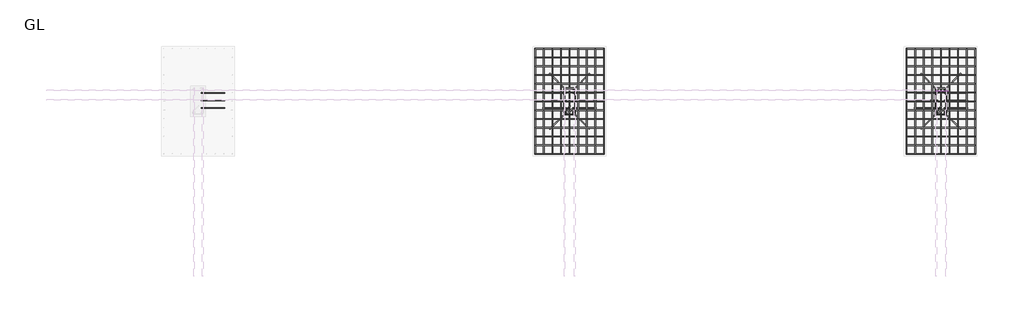
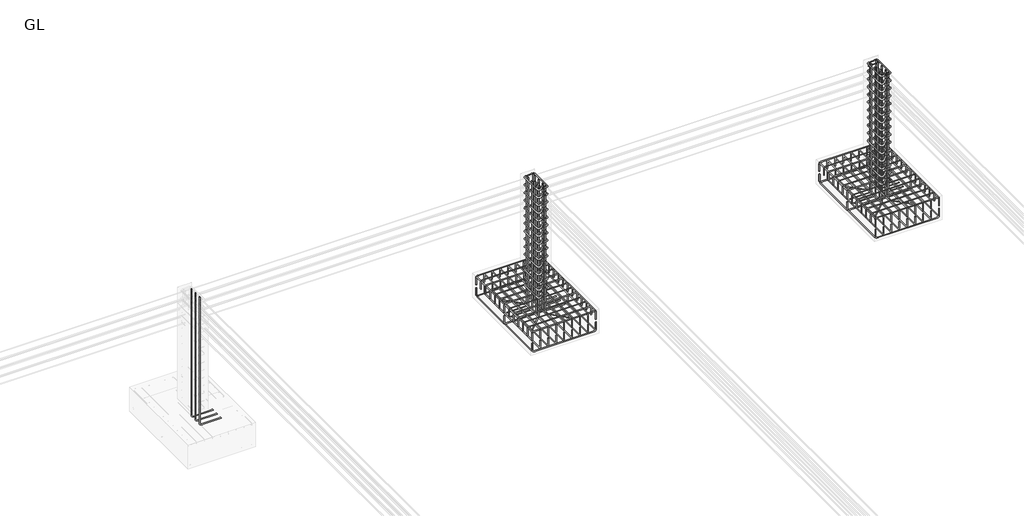
# One storey, part 16 of 16: 24 reinforcing bars.
"""IFC4 building model written with IfcOpenShell, lengths in millimetres."""

from ifc_helpers import new_model, si_unit, point, frame, origin, place, context, project, spatial, polyline, circle_curve, trimmed, segment, composite_curve, source, transform, mapped, element, save
from ifc_brep_helpers import swept_disk

model = new_model("IFC4")

# Units and contexts
model_context = context("Model", 3, world=origin())
ifc_project = project(units=[si_unit("LENGTHUNIT", "METRE", prefix="MILLI")], contexts=[model_context])

# Site, building, storey
site = spatial("IfcSite", under=ifc_project)
building = spatial("IfcBuilding", under=site)
storey = spatial("IfcBuildingStorey", under=building, Name="GL", Elevation=-1829.0)

# Reinforcing bars
placement = place(None, origin())
reinforcing_bar_shape = source(origin(), model_context, "Body", "SolidModel", [
    swept_disk(composite_curve([segment(polyline([(2141.0455621, 4968.8832479, -2089.0), (2141.0455621, 4968.8832479, -2213.0)]), True, "CONTINUOUS"), segment(trimmed(circle_curve(frame((2111.0455621, 4968.8832479, -2213.0), z_axis=(0.0, 1.0, 0.0), x_axis=(30.0, 0.0, 0.0)), 30.0), [point((2141.0455621, 4968.8832479, -2213.0))], [point((2111.0455621, 4968.8832479, -2243.0))], True, "CARTESIAN"), True, "CONTINUOUS"), segment(polyline([(2111.0455621, 4968.8832479, -2243.0), (1043.0455621, 4968.8832479, -2243.0)]), True, "CONTINUOUS"), segment(trimmed(circle_curve(frame((1043.0455621, 4968.8832479, -2213.0), z_axis=(0.0, 1.0, 0.0), x_axis=(0.0, 0.0, -30.0)), 30.0), [point((1043.0455621, 4968.8832479, -2243.0))], [point((1013.0455621, 4968.8832479, -2213.0))], True, "CARTESIAN"), True, "CONTINUOUS"), segment(polyline([(1013.0455621, 4968.8832479, -2213.0), (1013.0455621, 4968.8832479, -2089.0)]), True, "CONTINUOUS")], self_intersect=False), 6.0),
])
element("IfcReinforcingBar", 1, at=placement, inside=storey, context=model_context, shape_type="MappedRepresentation", body=[
    mapped(reinforcing_bar_shape, transform((0.0, 0.0, 0.0), x_axis=(1.0, 0.0, 0.0), y_axis=(0.0, 1.0, 0.0), z_axis=(0.0, 0.0, 1.0))),
    mapped(reinforcing_bar_shape, transform((0.0, -864.0, 0.0), x_axis=(1.0, 0.0, 0.0), y_axis=(0.0, 1.0, 0.0), z_axis=(0.0, 0.0, 1.0))),
    mapped(reinforcing_bar_shape, transform((0.0, -1728.0, 0.0), x_axis=(1.0, 0.0, 0.0), y_axis=(0.0, 1.0, 0.0), z_axis=(0.0, 0.0, 1.0))),
])
reinforcing_bar_2_shape = source(origin(), model_context, "Body", "SolidModel", [
    swept_disk(composite_curve([segment(polyline([(1013.0455621, 4968.8832479, -2022.436678), (1013.0455621, 4968.8832479, -1898.436678)]), True, "CONTINUOUS"), segment(trimmed(circle_curve(frame((1043.0455621, 4968.8832479, -1898.436678), z_axis=(0.0, 1.0, 0.0), x_axis=(-30.000000000000114, 0.0, 0.0)), 30.0), [point((1013.0455621, 4968.8832479, -1898.436678))], [point((1043.0455621, 4968.8832479, -1868.436678))], True, "CARTESIAN"), True, "CONTINUOUS"), segment(polyline([(1043.0455621, 4968.8832479, -1868.436678), (2111.0455621, 4968.8832479, -1868.436678)]), True, "CONTINUOUS"), segment(trimmed(circle_curve(frame((2111.0455621, 4968.8832479, -1898.436678), z_axis=(0.0, 1.0, 0.0), x_axis=(0.0, 0.0, 30.0)), 30.0), [point((2111.0455621, 4968.8832479, -1868.436678))], [point((2141.0455621, 4968.8832479, -1898.436678))], True, "CARTESIAN"), True, "CONTINUOUS"), segment(polyline([(2141.0455621, 4968.8832479, -1898.436678), (2141.0455621, 4968.8832479, -2022.436678)]), True, "CONTINUOUS")], self_intersect=False), 6.0),
])
element("IfcReinforcingBar", 2, at=placement, inside=storey, context=model_context, shape_type="MappedRepresentation", body=[
    mapped(reinforcing_bar_2_shape, transform((0.0, 0.0, 0.0), x_axis=(1.0, 0.0, 0.0), y_axis=(0.0, 1.0, 0.0), z_axis=(0.0, 0.0, 1.0))),
    mapped(reinforcing_bar_2_shape, transform((0.0, -144.0, 0.0), x_axis=(1.0, 0.0, 0.0), y_axis=(0.0, 1.0, 0.0), z_axis=(0.0, 0.0, 1.0))),
    mapped(reinforcing_bar_2_shape, transform((0.0, -288.0, 0.0), x_axis=(1.0, 0.0, 0.0), y_axis=(0.0, 1.0, 0.0), z_axis=(0.0, 0.0, 1.0))),
    mapped(reinforcing_bar_2_shape, transform((0.0, -432.0, 0.0), x_axis=(1.0, 0.0, 0.0), y_axis=(0.0, 1.0, 0.0), z_axis=(0.0, 0.0, 1.0))),
    mapped(reinforcing_bar_2_shape, transform((0.0, -576.0, 0.0), x_axis=(1.0, 0.0, 0.0), y_axis=(0.0, 1.0, 0.0), z_axis=(0.0, 0.0, 1.0))),
    mapped(reinforcing_bar_2_shape, transform((0.0, -720.0, 0.0), x_axis=(1.0, 0.0, 0.0), y_axis=(0.0, 1.0, 0.0), z_axis=(0.0, 0.0, 1.0))),
    mapped(reinforcing_bar_2_shape, transform((0.0, -864.0, 0.0), x_axis=(1.0, 0.0, 0.0), y_axis=(0.0, 1.0, 0.0), z_axis=(0.0, 0.0, 1.0))),
    mapped(reinforcing_bar_2_shape, transform((0.0, -1008.0, 0.0), x_axis=(1.0, 0.0, 0.0), y_axis=(0.0, 1.0, 0.0), z_axis=(0.0, 0.0, 1.0))),
    mapped(reinforcing_bar_2_shape, transform((0.0, -1152.0, 0.0), x_axis=(1.0, 0.0, 0.0), y_axis=(0.0, 1.0, 0.0), z_axis=(0.0, 0.0, 1.0))),
    mapped(reinforcing_bar_2_shape, transform((0.0, -1296.0, 0.0), x_axis=(1.0, 0.0, 0.0), y_axis=(0.0, 1.0, 0.0), z_axis=(0.0, 0.0, 1.0))),
    mapped(reinforcing_bar_2_shape, transform((0.0, -1440.0, 0.0), x_axis=(1.0, 0.0, 0.0), y_axis=(0.0, 1.0, 0.0), z_axis=(0.0, 0.0, 1.0))),
    mapped(reinforcing_bar_2_shape, transform((0.0, -1584.0, 0.0), x_axis=(1.0, 0.0, 0.0), y_axis=(0.0, 1.0, 0.0), z_axis=(0.0, 0.0, 1.0))),
    mapped(reinforcing_bar_2_shape, transform((0.0, -1728.0, 0.0), x_axis=(1.0, 0.0, 0.0), y_axis=(0.0, 1.0, 0.0), z_axis=(0.0, 0.0, 1.0))),
])
reinforcing_bar_3_shape = source(origin(), model_context, "Body", "SolidModel", [
    swept_disk(composite_curve([segment(polyline([(1013.0455621, 3240.8832479, -2027.5081232), (1013.0455621, 3240.8832479, -1903.5081232)]), True, "CONTINUOUS"), segment(trimmed(circle_curve(frame((1013.0455621, 3270.8832479, -1903.5081232), z_axis=(-1.0, 0.0, 0.0), x_axis=(0.0, -30.0, 0.0)), 30.0), [point((1013.0455621, 3240.8832479, -1903.5081232))], [point((1013.0455621, 3270.8832479, -1873.5081232))], True, "CARTESIAN"), True, "CONTINUOUS"), segment(polyline([(1013.0455621, 3270.8832479, -1873.5081232), (1013.0455621, 4938.8832479, -1873.5081232)]), True, "CONTINUOUS"), segment(trimmed(circle_curve(frame((1013.0455621, 4938.8832479, -1903.5081232), z_axis=(-1.0, 0.0, 0.0), x_axis=(0.0, 0.0, 30.0)), 30.0), [point((1013.0455621, 4938.8832479, -1873.5081232))], [point((1013.0455621, 4968.8832479, -1903.5081232))], True, "CARTESIAN"), True, "CONTINUOUS"), segment(polyline([(1013.0455621, 4968.8832479, -1903.5081232), (1013.0455621, 4968.8832479, -2027.5081232)]), True, "CONTINUOUS")], self_intersect=False), 6.0),
])
element("IfcReinforcingBar", 3, at=placement, inside=storey, context=model_context, shape_type="MappedRepresentation", body=[
    mapped(reinforcing_bar_3_shape, transform((0.0, 0.0, 0.0), x_axis=(1.0, 0.0, 0.0), y_axis=(0.0, 1.0, 0.0), z_axis=(0.0, 0.0, 1.0))),
    mapped(reinforcing_bar_3_shape, transform((141.0, 0.0, 0.0), x_axis=(1.0, 0.0, 0.0), y_axis=(0.0, 1.0, 0.0), z_axis=(0.0, 0.0, 1.0))),
    mapped(reinforcing_bar_3_shape, transform((282.0, 0.0, 0.0), x_axis=(1.0, 0.0, 0.0), y_axis=(0.0, 1.0, 0.0), z_axis=(0.0, 0.0, 1.0))),
    mapped(reinforcing_bar_3_shape, transform((423.0, 0.0, 0.0), x_axis=(1.0, 0.0, 0.0), y_axis=(0.0, 1.0, 0.0), z_axis=(0.0, 0.0, 1.0))),
    mapped(reinforcing_bar_3_shape, transform((564.0, 0.0, 0.0), x_axis=(1.0, 0.0, 0.0), y_axis=(0.0, 1.0, 0.0), z_axis=(0.0, 0.0, 1.0))),
    mapped(reinforcing_bar_3_shape, transform((705.0, 0.0, 0.0), x_axis=(1.0, 0.0, 0.0), y_axis=(0.0, 1.0, 0.0), z_axis=(0.0, 0.0, 1.0))),
    mapped(reinforcing_bar_3_shape, transform((846.0, 0.0, 0.0), x_axis=(1.0, 0.0, 0.0), y_axis=(0.0, 1.0, 0.0), z_axis=(0.0, 0.0, 1.0))),
    mapped(reinforcing_bar_3_shape, transform((987.0, 0.0, 0.0), x_axis=(1.0, 0.0, 0.0), y_axis=(0.0, 1.0, 0.0), z_axis=(0.0, 0.0, 1.0))),
    mapped(reinforcing_bar_3_shape, transform((1128.0, 0.0, 0.0), x_axis=(1.0, 0.0, 0.0), y_axis=(0.0, 1.0, 0.0), z_axis=(0.0, 0.0, 1.0))),
])
reinforcing_bar_4_shape = source(origin(), model_context, "Body", "SolidModel", [
    swept_disk(composite_curve([segment(polyline([(2141.0455621, 3240.8832479, -2080.6239909), (2141.0455621, 3240.8832479, -2204.6239909)]), True, "CONTINUOUS"), segment(trimmed(circle_curve(frame((2141.0455621, 3270.8832479, -2204.6239909), z_axis=(1.0, 0.0, 0.0), x_axis=(0.0, -30.0, 0.0)), 30.0), [point((2141.0455621, 3240.8832479, -2204.6239909))], [point((2141.0455621, 3270.8832479, -2234.6239909))], True, "CARTESIAN"), True, "CONTINUOUS"), segment(polyline([(2141.0455621, 3270.8832479, -2234.6239909), (2141.0455621, 4925.8578108, -2234.6239909)]), True, "CONTINUOUS"), segment(trimmed(circle_curve(frame((2141.0455621, 4925.8578108, -2204.6239909), z_axis=(1.0, 0.0, 0.0), x_axis=(0.0, 0.0, -30.0)), 30.0), [point((2141.0455621, 4925.8578108, -2234.6239909))], [point((2141.0455621, 4955.8578108, -2204.6239909))], True, "CARTESIAN"), True, "CONTINUOUS"), segment(polyline([(2141.0455621, 4955.8578108, -2204.6239909), (2141.0455621, 4955.8578108, -2080.6239909)]), True, "CONTINUOUS")], self_intersect=False), 6.0),
])
element("IfcReinforcingBar", 4, at=placement, inside=storey, context=model_context, shape_type="MappedRepresentation", body=[
    mapped(reinforcing_bar_4_shape, transform((0.0, 0.0, 0.0), x_axis=(1.0, 0.0, 0.0), y_axis=(0.0, 1.0, 0.0), z_axis=(0.0, 0.0, 1.0))),
    mapped(reinforcing_bar_4_shape, transform((-141.0, 0.0, 0.0), x_axis=(1.0, 0.0, 0.0), y_axis=(0.0, 1.0, 0.0), z_axis=(0.0, 0.0, 1.0))),
    mapped(reinforcing_bar_4_shape, transform((-282.0, 0.0, 0.0), x_axis=(1.0, 0.0, 0.0), y_axis=(0.0, 1.0, 0.0), z_axis=(0.0, 0.0, 1.0))),
    mapped(reinforcing_bar_4_shape, transform((-423.0, 0.0, 0.0), x_axis=(1.0, 0.0, 0.0), y_axis=(0.0, 1.0, 0.0), z_axis=(0.0, 0.0, 1.0))),
    mapped(reinforcing_bar_4_shape, transform((-564.0, 0.0, 0.0), x_axis=(1.0, 0.0, 0.0), y_axis=(0.0, 1.0, 0.0), z_axis=(0.0, 0.0, 1.0))),
    mapped(reinforcing_bar_4_shape, transform((-705.0, 0.0, 0.0), x_axis=(1.0, 0.0, 0.0), y_axis=(0.0, 1.0, 0.0), z_axis=(0.0, 0.0, 1.0))),
    mapped(reinforcing_bar_4_shape, transform((-846.0, 0.0, 0.0), x_axis=(1.0, 0.0, 0.0), y_axis=(0.0, 1.0, 0.0), z_axis=(0.0, 0.0, 1.0))),
    mapped(reinforcing_bar_4_shape, transform((-987.0, 0.0, 0.0), x_axis=(1.0, 0.0, 0.0), y_axis=(0.0, 1.0, 0.0), z_axis=(0.0, 0.0, 1.0))),
    mapped(reinforcing_bar_4_shape, transform((-1128.0, 0.0, 0.0), x_axis=(1.0, 0.0, 0.0), y_axis=(0.0, 1.0, 0.0), z_axis=(0.0, 0.0, 1.0))),
])
reinforcing_bar_5_shape = source(origin(), model_context, "Body", "SolidModel", [
    swept_disk(composite_curve([segment(polyline([(8237.0455621, 4968.8832479, -2089.0), (8237.0455621, 4968.8832479, -2213.0)]), True, "CONTINUOUS"), segment(trimmed(circle_curve(frame((8207.0455621, 4968.8832479, -2213.0), z_axis=(0.0, 1.0, 0.0), x_axis=(30.0, 0.0, 0.0)), 30.0), [point((8237.0455621, 4968.8832479, -2213.0))], [point((8207.0455621, 4968.8832479, -2243.0))], True, "CARTESIAN"), True, "CONTINUOUS"), segment(polyline([(8207.0455621, 4968.8832479, -2243.0), (7139.0455621, 4968.8832479, -2243.0)]), True, "CONTINUOUS"), segment(trimmed(circle_curve(frame((7139.0455621, 4968.8832479, -2213.0), z_axis=(0.0, 1.0, 0.0), x_axis=(0.0, 0.0, -30.0)), 30.0), [point((7139.0455621, 4968.8832479, -2243.0))], [point((7109.0455621, 4968.8832479, -2213.0))], True, "CARTESIAN"), True, "CONTINUOUS"), segment(polyline([(7109.0455621, 4968.8832479, -2213.0), (7109.0455621, 4968.8832479, -2089.0)]), True, "CONTINUOUS")], self_intersect=False), 6.0),
])
element("IfcReinforcingBar", 5, at=placement, inside=storey, context=model_context, shape_type="MappedRepresentation", body=[
    mapped(reinforcing_bar_5_shape, transform((0.0, 0.0, 0.0), x_axis=(1.0, 0.0, 0.0), y_axis=(0.0, 1.0, 0.0), z_axis=(0.0, 0.0, 1.0))),
    mapped(reinforcing_bar_5_shape, transform((0.0, -864.0, 0.0), x_axis=(1.0, 0.0, 0.0), y_axis=(0.0, 1.0, 0.0), z_axis=(0.0, 0.0, 1.0))),
    mapped(reinforcing_bar_5_shape, transform((0.0, -1728.0, 0.0), x_axis=(1.0, 0.0, 0.0), y_axis=(0.0, 1.0, 0.0), z_axis=(0.0, 0.0, 1.0))),
])
reinforcing_bar_6_shape = source(origin(), model_context, "Body", "SolidModel", [
    swept_disk(composite_curve([segment(polyline([(7109.0455621, 4968.8832479, -2022.436678), (7109.0455621, 4968.8832479, -1898.436678)]), True, "CONTINUOUS"), segment(trimmed(circle_curve(frame((7139.0455621, 4968.8832479, -1898.436678), z_axis=(0.0, 1.0, 0.0), x_axis=(-30.0, 0.0, 0.0)), 30.0), [point((7109.0455621, 4968.8832479, -1898.436678))], [point((7139.0455621, 4968.8832479, -1868.436678))], True, "CARTESIAN"), True, "CONTINUOUS"), segment(polyline([(7139.0455621, 4968.8832479, -1868.436678), (8207.0455621, 4968.8832479, -1868.436678)]), True, "CONTINUOUS"), segment(trimmed(circle_curve(frame((8207.0455621, 4968.8832479, -1898.436678), z_axis=(0.0, 1.0, 0.0), x_axis=(0.0, 0.0, 30.0)), 30.0), [point((8207.0455621, 4968.8832479, -1868.436678))], [point((8237.0455621, 4968.8832479, -1898.436678))], True, "CARTESIAN"), True, "CONTINUOUS"), segment(polyline([(8237.0455621, 4968.8832479, -1898.436678), (8237.0455621, 4968.8832479, -2022.436678)]), True, "CONTINUOUS")], self_intersect=False), 6.0),
])
element("IfcReinforcingBar", 6, at=placement, inside=storey, context=model_context, shape_type="MappedRepresentation", body=[
    mapped(reinforcing_bar_6_shape, transform((0.0, 0.0, 0.0), x_axis=(1.0, 0.0, 0.0), y_axis=(0.0, 1.0, 0.0), z_axis=(0.0, 0.0, 1.0))),
    mapped(reinforcing_bar_6_shape, transform((0.0, -144.0, 0.0), x_axis=(1.0, 0.0, 0.0), y_axis=(0.0, 1.0, 0.0), z_axis=(0.0, 0.0, 1.0))),
    mapped(reinforcing_bar_6_shape, transform((0.0, -288.0, 0.0), x_axis=(1.0, 0.0, 0.0), y_axis=(0.0, 1.0, 0.0), z_axis=(0.0, 0.0, 1.0))),
    mapped(reinforcing_bar_6_shape, transform((0.0, -432.0, 0.0), x_axis=(1.0, 0.0, 0.0), y_axis=(0.0, 1.0, 0.0), z_axis=(0.0, 0.0, 1.0))),
    mapped(reinforcing_bar_6_shape, transform((0.0, -576.0, 0.0), x_axis=(1.0, 0.0, 0.0), y_axis=(0.0, 1.0, 0.0), z_axis=(0.0, 0.0, 1.0))),
    mapped(reinforcing_bar_6_shape, transform((0.0, -720.0, 0.0), x_axis=(1.0, 0.0, 0.0), y_axis=(0.0, 1.0, 0.0), z_axis=(0.0, 0.0, 1.0))),
    mapped(reinforcing_bar_6_shape, transform((0.0, -864.0, 0.0), x_axis=(1.0, 0.0, 0.0), y_axis=(0.0, 1.0, 0.0), z_axis=(0.0, 0.0, 1.0))),
    mapped(reinforcing_bar_6_shape, transform((0.0, -1008.0, 0.0), x_axis=(1.0, 0.0, 0.0), y_axis=(0.0, 1.0, 0.0), z_axis=(0.0, 0.0, 1.0))),
    mapped(reinforcing_bar_6_shape, transform((0.0, -1152.0, 0.0), x_axis=(1.0, 0.0, 0.0), y_axis=(0.0, 1.0, 0.0), z_axis=(0.0, 0.0, 1.0))),
    mapped(reinforcing_bar_6_shape, transform((0.0, -1296.0, 0.0), x_axis=(1.0, 0.0, 0.0), y_axis=(0.0, 1.0, 0.0), z_axis=(0.0, 0.0, 1.0))),
    mapped(reinforcing_bar_6_shape, transform((0.0, -1440.0, 0.0), x_axis=(1.0, 0.0, 0.0), y_axis=(0.0, 1.0, 0.0), z_axis=(0.0, 0.0, 1.0))),
    mapped(reinforcing_bar_6_shape, transform((0.0, -1584.0, 0.0), x_axis=(1.0, 0.0, 0.0), y_axis=(0.0, 1.0, 0.0), z_axis=(0.0, 0.0, 1.0))),
    mapped(reinforcing_bar_6_shape, transform((0.0, -1728.0, 0.0), x_axis=(1.0, 0.0, 0.0), y_axis=(0.0, 1.0, 0.0), z_axis=(0.0, 0.0, 1.0))),
])
reinforcing_bar_7_shape = source(origin(), model_context, "Body", "SolidModel", [
    swept_disk(composite_curve([segment(polyline([(7109.0455621, 3240.8832479, -2027.5081232), (7109.0455621, 3240.8832479, -1903.5081232)]), True, "CONTINUOUS"), segment(trimmed(circle_curve(frame((7109.0455621, 3270.8832479, -1903.5081232), z_axis=(-1.0, 0.0, 0.0), x_axis=(0.0, -30.0, 0.0)), 30.0), [point((7109.0455621, 3240.8832479, -1903.5081232))], [point((7109.0455621, 3270.8832479, -1873.5081232))], True, "CARTESIAN"), True, "CONTINUOUS"), segment(polyline([(7109.0455621, 3270.8832479, -1873.5081232), (7109.0455621, 4938.8832479, -1873.5081232)]), True, "CONTINUOUS"), segment(trimmed(circle_curve(frame((7109.0455621, 4938.8832479, -1903.5081232), z_axis=(-1.0, 0.0, 0.0), x_axis=(0.0, 0.0, 30.0)), 30.0), [point((7109.0455621, 4938.8832479, -1873.5081232))], [point((7109.0455621, 4968.8832479, -1903.5081232))], True, "CARTESIAN"), True, "CONTINUOUS"), segment(polyline([(7109.0455621, 4968.8832479, -1903.5081232), (7109.0455621, 4968.8832479, -2027.5081232)]), True, "CONTINUOUS")], self_intersect=False), 6.0),
])
element("IfcReinforcingBar", 7, at=placement, inside=storey, context=model_context, shape_type="MappedRepresentation", body=[
    mapped(reinforcing_bar_7_shape, transform((0.0, 0.0, 0.0), x_axis=(1.0, 0.0, 0.0), y_axis=(0.0, 1.0, 0.0), z_axis=(0.0, 0.0, 1.0))),
    mapped(reinforcing_bar_7_shape, transform((141.0, 0.0, 0.0), x_axis=(1.0, 0.0, 0.0), y_axis=(0.0, 1.0, 0.0), z_axis=(0.0, 0.0, 1.0))),
    mapped(reinforcing_bar_7_shape, transform((282.0, 0.0, 0.0), x_axis=(1.0, 0.0, 0.0), y_axis=(0.0, 1.0, 0.0), z_axis=(0.0, 0.0, 1.0))),
    mapped(reinforcing_bar_7_shape, transform((423.0, 0.0, 0.0), x_axis=(1.0, 0.0, 0.0), y_axis=(0.0, 1.0, 0.0), z_axis=(0.0, 0.0, 1.0))),
    mapped(reinforcing_bar_7_shape, transform((564.0, 0.0, 0.0), x_axis=(1.0, 0.0, 0.0), y_axis=(0.0, 1.0, 0.0), z_axis=(0.0, 0.0, 1.0))),
    mapped(reinforcing_bar_7_shape, transform((705.0, 0.0, 0.0), x_axis=(1.0, 0.0, 0.0), y_axis=(0.0, 1.0, 0.0), z_axis=(0.0, 0.0, 1.0))),
    mapped(reinforcing_bar_7_shape, transform((846.0, 0.0, 0.0), x_axis=(1.0, 0.0, 0.0), y_axis=(0.0, 1.0, 0.0), z_axis=(0.0, 0.0, 1.0))),
    mapped(reinforcing_bar_7_shape, transform((987.0, 0.0, 0.0), x_axis=(1.0, 0.0, 0.0), y_axis=(0.0, 1.0, 0.0), z_axis=(0.0, 0.0, 1.0))),
    mapped(reinforcing_bar_7_shape, transform((1128.0, 0.0, 0.0), x_axis=(1.0, 0.0, 0.0), y_axis=(0.0, 1.0, 0.0), z_axis=(0.0, 0.0, 1.0))),
])
reinforcing_bar_8_shape = source(origin(), model_context, "Body", "SolidModel", [
    swept_disk(composite_curve([segment(polyline([(8237.0455621, 3240.8832479, -2080.6239909), (8237.0455621, 3240.8832479, -2204.6239909)]), True, "CONTINUOUS"), segment(trimmed(circle_curve(frame((8237.0455621, 3270.8832479, -2204.6239909), z_axis=(1.0, 0.0, 0.0), x_axis=(0.0, -30.0, 0.0)), 30.0), [point((8237.0455621, 3240.8832479, -2204.6239909))], [point((8237.0455621, 3270.8832479, -2234.6239909))], True, "CARTESIAN"), True, "CONTINUOUS"), segment(polyline([(8237.0455621, 3270.8832479, -2234.6239909), (8237.0455621, 4925.8578108, -2234.6239909)]), True, "CONTINUOUS"), segment(trimmed(circle_curve(frame((8237.0455621, 4925.8578108, -2204.6239909), z_axis=(1.0, 0.0, 0.0), x_axis=(0.0, 0.0, -30.0)), 30.0), [point((8237.0455621, 4925.8578108, -2234.6239909))], [point((8237.0455621, 4955.8578108, -2204.6239909))], True, "CARTESIAN"), True, "CONTINUOUS"), segment(polyline([(8237.0455621, 4955.8578108, -2204.6239909), (8237.0455621, 4955.8578108, -2080.6239909)]), True, "CONTINUOUS")], self_intersect=False), 6.0),
])
element("IfcReinforcingBar", 8, at=placement, inside=storey, context=model_context, shape_type="MappedRepresentation", body=[
    mapped(reinforcing_bar_8_shape, transform((0.0, 0.0, 0.0), x_axis=(1.0, 0.0, 0.0), y_axis=(0.0, 1.0, 0.0), z_axis=(0.0, 0.0, 1.0))),
    mapped(reinforcing_bar_8_shape, transform((-141.0, 0.0, 0.0), x_axis=(1.0, 0.0, 0.0), y_axis=(0.0, 1.0, 0.0), z_axis=(0.0, 0.0, 1.0))),
    mapped(reinforcing_bar_8_shape, transform((-282.0, 0.0, 0.0), x_axis=(1.0, 0.0, 0.0), y_axis=(0.0, 1.0, 0.0), z_axis=(0.0, 0.0, 1.0))),
    mapped(reinforcing_bar_8_shape, transform((-423.0, 0.0, 0.0), x_axis=(1.0, 0.0, 0.0), y_axis=(0.0, 1.0, 0.0), z_axis=(0.0, 0.0, 1.0))),
    mapped(reinforcing_bar_8_shape, transform((-564.0, 0.0, 0.0), x_axis=(1.0, 0.0, 0.0), y_axis=(0.0, 1.0, 0.0), z_axis=(0.0, 0.0, 1.0))),
    mapped(reinforcing_bar_8_shape, transform((-705.0, 0.0, 0.0), x_axis=(1.0, 0.0, 0.0), y_axis=(0.0, 1.0, 0.0), z_axis=(0.0, 0.0, 1.0))),
    mapped(reinforcing_bar_8_shape, transform((-846.0, 0.0, 0.0), x_axis=(1.0, 0.0, 0.0), y_axis=(0.0, 1.0, 0.0), z_axis=(0.0, 0.0, 1.0))),
    mapped(reinforcing_bar_8_shape, transform((-987.0, 0.0, 0.0), x_axis=(1.0, 0.0, 0.0), y_axis=(0.0, 1.0, 0.0), z_axis=(0.0, 0.0, 1.0))),
    mapped(reinforcing_bar_8_shape, transform((-1128.0, 0.0, 0.0), x_axis=(1.0, 0.0, 0.0), y_axis=(0.0, 1.0, 0.0), z_axis=(0.0, 0.0, 1.0))),
])
reinforcing_bar_9_shape = source(origin(), model_context, "Body", "SolidModel", [
    swept_disk(composite_curve([segment(polyline([(-4461.8446527, 3997.0882595, 241.0), (-4461.8446527, 3997.0882595, -2129.0)]), True, "CONTINUOUS"), segment(trimmed(circle_curve(frame((-4431.8446527, 3997.0882595, -2129.0), z_axis=(0.0, -1.0, 0.0), x_axis=(-30.0, 0.0, 0.0)), 30.0), [point((-4461.8446527, 3997.0882595, -2129.0))], [point((-4431.8446527, 3997.0882595, -2159.0))], True, "CARTESIAN"), True, "CONTINUOUS"), segment(polyline([(-4431.8446527, 3997.0882595, -2159.0), (-4081.8446527, 3997.0882595, -2159.0)]), True, "CONTINUOUS")], self_intersect=False), 6.0),
])
element("IfcReinforcingBar", 9, at=placement, inside=storey, context=model_context, shape_type="MappedRepresentation", body=[
    mapped(reinforcing_bar_9_shape, transform((0.0, 0.0, 0.0), x_axis=(1.0, 0.0, 0.0), y_axis=(0.0, 1.0, 0.0), z_axis=(0.0, 0.0, 1.0))),
    mapped(reinforcing_bar_9_shape, transform((0.0, 123.5823926, 0.0), x_axis=(1.0, 0.0, 0.0), y_axis=(0.0, 1.0, 0.0), z_axis=(0.0, 0.0, 1.0))),
    mapped(reinforcing_bar_9_shape, transform((0.0, 247.1647853, 0.0), x_axis=(1.0, 0.0, 0.0), y_axis=(0.0, 1.0, 0.0), z_axis=(0.0, 0.0, 1.0))),
])
reinforcing_bar_10_shape = source(origin(), model_context, "Body", "SolidModel", [
    swept_disk(composite_curve([segment(polyline([(1584.5135995, 4029.7776922, -1793.0), (1496.8323586, 3942.0964514, -1793.0)]), True, "CONTINUOUS"), segment(trimmed(circle_curve(frame((1518.0455621, 3920.8832479, -1793.0), z_axis=(0.0, 0.0, 1.0), x_axis=(-21.21320350000019, 21.213203500000418, 0.0)), 30.0), [point((1496.8323586, 3942.0964514, -1793.0))], [point((1518.0455621, 3890.8832479, -1793.0))], True, "CARTESIAN"), True, "CONTINUOUS"), segment(polyline([(1518.0455621, 3890.8832479, -1793.0), (1636.0455621, 3890.8832479, -1793.0)]), True, "CONTINUOUS"), segment(trimmed(circle_curve(frame((1636.0455621, 3920.8832479, -1793.0), z_axis=(0.0, 0.0, 1.0), x_axis=(0.0, -30.0, 0.0)), 30.0), [point((1636.0455621, 3890.8832479, -1793.0))], [point((1666.0455621, 3920.8832479, -1793.0))], True, "CARTESIAN"), True, "CONTINUOUS"), segment(polyline([(1666.0455621, 3920.8832479, -1793.0), (1666.0455621, 4288.8832479, -1793.0)]), True, "CONTINUOUS"), segment(trimmed(circle_curve(frame((1636.1135038, 4288.8832479, -1795.0178916), z_axis=(-0.06726305234213417, 0.0, 0.9977352764083365), x_axis=(29.932058300000108, 0.0, 2.0178915999999845)), 30.0), [point((1666.0455621, 4288.8832479, -1793.0))], [point((1636.1135038, 4318.8832479, -1795.0178916))], True, "CARTESIAN"), True, "CONTINUOUS"), segment(polyline([(1636.1135038, 4318.8832479, -1795.0178916), (1517.9776204, 4318.8832479, -1802.9821084)]), True, "CONTINUOUS"), segment(trimmed(circle_curve(frame((1517.9776204, 4288.8832479, -1802.9821084), z_axis=(-0.06726305234213417, 0.0, 0.9977352764083365), x_axis=(0.0, 30.0, 0.0)), 30.0), [point((1517.9776204, 4318.8832479, -1802.9821084))], [point((1488.0455621, 4288.8832479, -1805.0))], True, "CARTESIAN"), True, "CONTINUOUS"), segment(polyline([(1488.0455621, 4288.8832479, -1805.0), (1488.0455621, 3920.8832479, -1805.0)]), True, "CONTINUOUS"), segment(trimmed(circle_curve(frame((1518.0455621, 3920.8832479, -1805.0), z_axis=(0.0, 0.0, 1.0), x_axis=(-30.0, 0.0, 0.0)), 30.0), [point((1488.0455621, 3920.8832479, -1805.0))], [point((1539.2587655, 3899.6700445, -1805.0))], True, "CARTESIAN"), True, "CONTINUOUS"), segment(polyline([(1539.2587655, 3899.6700445, -1805.0), (1626.9400064, 3987.3512854, -1805.0)]), True, "CONTINUOUS")], self_intersect=False), 6.0),
])
element("IfcReinforcingBar", 10, at=placement, inside=storey, context=model_context, shape_type="MappedRepresentation", body=[
    mapped(reinforcing_bar_10_shape, transform((0.0, 0.0, 0.0), x_axis=(1.0, 0.0, 0.0), y_axis=(0.0, 1.0, 0.0), z_axis=(0.0, 0.0, 1.0))),
    mapped(reinforcing_bar_10_shape, transform((0.0, 0.0, 144.8571429), x_axis=(1.0, 0.0, 0.0), y_axis=(0.0, 1.0, 0.0), z_axis=(0.0, 0.0, 1.0))),
    mapped(reinforcing_bar_10_shape, transform((0.0, 0.0, 289.7142857), x_axis=(1.0, 0.0, 0.0), y_axis=(0.0, 1.0, 0.0), z_axis=(0.0, 0.0, 1.0))),
    mapped(reinforcing_bar_10_shape, transform((0.0, 0.0, 434.5714286), x_axis=(1.0, 0.0, 0.0), y_axis=(0.0, 1.0, 0.0), z_axis=(0.0, 0.0, 1.0))),
    mapped(reinforcing_bar_10_shape, transform((0.0, 0.0, 579.4285714), x_axis=(1.0, 0.0, 0.0), y_axis=(0.0, 1.0, 0.0), z_axis=(0.0, 0.0, 1.0))),
    mapped(reinforcing_bar_10_shape, transform((0.0, 0.0, 724.2857143), x_axis=(1.0, 0.0, 0.0), y_axis=(0.0, 1.0, 0.0), z_axis=(0.0, 0.0, 1.0))),
    mapped(reinforcing_bar_10_shape, transform((0.0, 0.0, 869.1428571), x_axis=(1.0, 0.0, 0.0), y_axis=(0.0, 1.0, 0.0), z_axis=(0.0, 0.0, 1.0))),
    mapped(reinforcing_bar_10_shape, transform((0.0, 0.0, 1014.0), x_axis=(1.0, 0.0, 0.0), y_axis=(0.0, 1.0, 0.0), z_axis=(0.0, 0.0, 1.0))),
    mapped(reinforcing_bar_10_shape, transform((0.0, 0.0, 1158.8571429), x_axis=(1.0, 0.0, 0.0), y_axis=(0.0, 1.0, 0.0), z_axis=(0.0, 0.0, 1.0))),
    mapped(reinforcing_bar_10_shape, transform((0.0, 0.0, 1303.7142857), x_axis=(1.0, 0.0, 0.0), y_axis=(0.0, 1.0, 0.0), z_axis=(0.0, 0.0, 1.0))),
    mapped(reinforcing_bar_10_shape, transform((0.0, 0.0, 1448.5714286), x_axis=(1.0, 0.0, 0.0), y_axis=(0.0, 1.0, 0.0), z_axis=(0.0, 0.0, 1.0))),
    mapped(reinforcing_bar_10_shape, transform((0.0, 0.0, 1593.4285714), x_axis=(1.0, 0.0, 0.0), y_axis=(0.0, 1.0, 0.0), z_axis=(0.0, 0.0, 1.0))),
    mapped(reinforcing_bar_10_shape, transform((0.0, 0.0, 1738.2857143), x_axis=(1.0, 0.0, 0.0), y_axis=(0.0, 1.0, 0.0), z_axis=(0.0, 0.0, 1.0))),
    mapped(reinforcing_bar_10_shape, transform((0.0, 0.0, 1883.1428571), x_axis=(1.0, 0.0, 0.0), y_axis=(0.0, 1.0, 0.0), z_axis=(0.0, 0.0, 1.0))),
    mapped(reinforcing_bar_10_shape, transform((0.0, 0.0, 2028.0), x_axis=(1.0, 0.0, 0.0), y_axis=(0.0, 1.0, 0.0), z_axis=(0.0, 0.0, 1.0))),
])
element("IfcReinforcingBar", 11, at=placement, inside=storey, context=model_context, shape_type="SolidModel", body=[
    swept_disk(composite_curve([segment(polyline([(1519.9357768, 3919.9357561, 241.0), (1519.9357768, 3919.9357561, -2129.0)]), True, "CONTINUOUS"), segment(trimmed(circle_curve(frame((1498.7225734, 3898.7225527, -2129.0), z_axis=(-0.7071067811865187, 0.7071067811865764, 0.0), x_axis=(21.213203399999884, 21.21320340000011, 0.0)), 30.0), [point((1519.9357768, 3919.9357561, -2129.0))], [point((1498.7225734, 3898.7225527, -2159.0))], True, "CARTESIAN"), True, "CONTINUOUS"), segment(polyline([(1498.7225734, 3898.7225527, -2159.0), (1251.2352, 3651.2351793, -2159.0)]), True, "CONTINUOUS")], self_intersect=False), 6.0),
])
element("IfcReinforcingBar", 12, at=placement, inside=storey, context=model_context, shape_type="SolidModel", body=[
    swept_disk(composite_curve([segment(polyline([(1519.9357768, 4289.8307397, 241.0), (1519.9357768, 4289.8307397, -2129.0)]), True, "CONTINUOUS"), segment(trimmed(circle_curve(frame((1498.7225734, 4311.0439432, -2129.0), z_axis=(0.7071067811865218, 0.7071067811865733, 0.0), x_axis=(21.213203399999884, -21.213203500000418, 0.0)), 30.0), [point((1519.9357768, 4289.8307397, -2129.0))], [point((1498.7225734, 4311.0439432, -2159.0))], True, "CARTESIAN"), True, "CONTINUOUS"), segment(polyline([(1498.7225734, 4311.0439432, -2159.0), (1251.2352, 4558.5313166, -2159.0)]), True, "CONTINUOUS")], self_intersect=False), 6.0),
])
element("IfcReinforcingBar", 13, at=placement, inside=storey, context=model_context, shape_type="SolidModel", body=[
    swept_disk(composite_curve([segment(polyline([(1634.1553473, 3919.9357561, 241.0), (1634.1553473, 3919.9357561, -2129.0)]), True, "CONTINUOUS"), segment(trimmed(circle_curve(frame((1655.3685508, 3898.7225527, -2129.0), z_axis=(-0.7071067811865248, -0.7071067811865703, 0.0), x_axis=(-21.21320350000019, 21.21320340000011, 0.0)), 30.0), [point((1634.1553473, 3919.9357561, -2129.0))], [point((1655.3685508, 3898.7225527, -2159.0))], True, "CARTESIAN"), True, "CONTINUOUS"), segment(polyline([(1655.3685508, 3898.7225527, -2159.0), (1902.8559242, 3651.2351793, -2159.0)]), True, "CONTINUOUS")], self_intersect=False), 6.0),
])
element("IfcReinforcingBar", 14, at=placement, inside=storey, context=model_context, shape_type="SolidModel", body=[
    swept_disk(composite_curve([segment(polyline([(1634.1553473, 4289.8307397, 241.0), (1634.1553473, 4289.8307397, -2129.0)]), True, "CONTINUOUS"), segment(trimmed(circle_curve(frame((1655.3685508, 4311.0439432, -2129.0), z_axis=(0.7071067811865157, -0.7071067811865794, 0.0), x_axis=(-21.21320350000019, -21.213203500000418, 0.0)), 30.0), [point((1634.1553473, 4289.8307397, -2129.0))], [point((1655.3685508, 4311.0439432, -2159.0))], True, "CARTESIAN"), True, "CONTINUOUS"), segment(polyline([(1655.3685508, 4311.0439432, -2159.0), (1902.8559242, 4558.5313166, -2159.0)]), True, "CONTINUOUS")], self_intersect=False), 6.0),
])
reinforcing_bar_11_shape = source(origin(), model_context, "Body", "SolidModel", [
    swept_disk(composite_curve([segment(polyline([(1519.9357768, 3997.0882595, 241.0), (1519.9357768, 3997.0882595, -2129.0)]), True, "CONTINUOUS"), segment(trimmed(circle_curve(frame((1489.9357768, 3997.0882595, -2129.0), z_axis=(0.0, 1.0, 0.0), x_axis=(30.0, 0.0, 0.0)), 30.0), [point((1519.9357768, 3997.0882595, -2129.0))], [point((1489.9357768, 3997.0882595, -2159.0))], True, "CARTESIAN"), True, "CONTINUOUS"), segment(polyline([(1489.9357768, 3997.0882595, -2159.0), (1139.9357768, 3997.0882595, -2159.0)]), True, "CONTINUOUS")], self_intersect=False), 6.0),
])
element("IfcReinforcingBar", 15, at=placement, inside=storey, context=model_context, shape_type="MappedRepresentation", body=[
    mapped(reinforcing_bar_11_shape, transform((0.0, 0.0, 0.0), x_axis=(1.0, 0.0, 0.0), y_axis=(0.0, 1.0, 0.0), z_axis=(0.0, 0.0, 1.0))),
    mapped(reinforcing_bar_11_shape, transform((0.0, 123.5823926, 0.0), x_axis=(1.0, 0.0, 0.0), y_axis=(0.0, 1.0, 0.0), z_axis=(0.0, 0.0, 1.0))),
    mapped(reinforcing_bar_11_shape, transform((0.0, 247.1647853, 0.0), x_axis=(1.0, 0.0, 0.0), y_axis=(0.0, 1.0, 0.0), z_axis=(0.0, 0.0, 1.0))),
])
reinforcing_bar_12_shape = source(origin(), model_context, "Body", "SolidModel", [
    swept_disk(composite_curve([segment(polyline([(1634.1553473, 3997.0882595, 241.0), (1634.1553473, 3997.0882595, -2129.0)]), True, "CONTINUOUS"), segment(trimmed(circle_curve(frame((1664.1553473, 3997.0882595, -2129.0), z_axis=(0.0, -1.0, 0.0), x_axis=(-30.0, 0.0, 0.0)), 30.0), [point((1634.1553473, 3997.0882595, -2129.0))], [point((1664.1553473, 3997.0882595, -2159.0))], True, "CARTESIAN"), True, "CONTINUOUS"), segment(polyline([(1664.1553473, 3997.0882595, -2159.0), (2014.1553473, 3997.0882595, -2159.0)]), True, "CONTINUOUS")], self_intersect=False), 6.0),
])
element("IfcReinforcingBar", 16, at=placement, inside=storey, context=model_context, shape_type="MappedRepresentation", body=[
    mapped(reinforcing_bar_12_shape, transform((0.0, 0.0, 0.0), x_axis=(1.0, 0.0, 0.0), y_axis=(0.0, 1.0, 0.0), z_axis=(0.0, 0.0, 1.0))),
    mapped(reinforcing_bar_12_shape, transform((0.0, 123.5823926, 0.0), x_axis=(1.0, 0.0, 0.0), y_axis=(0.0, 1.0, 0.0), z_axis=(0.0, 0.0, 1.0))),
    mapped(reinforcing_bar_12_shape, transform((0.0, 247.1647853, 0.0), x_axis=(1.0, 0.0, 0.0), y_axis=(0.0, 1.0, 0.0), z_axis=(0.0, 0.0, 1.0))),
])
reinforcing_bar_13_shape = source(origin(), model_context, "Body", "SolidModel", [
    swept_disk(composite_curve([segment(polyline([(7680.5135995, 4029.7776922, -1793.0), (7592.8323586, 3942.0964514, -1793.0)]), True, "CONTINUOUS"), segment(trimmed(circle_curve(frame((7614.0455621, 3920.8832479, -1793.0), z_axis=(0.0, 0.0, 1.0), x_axis=(-21.213203500000418, 21.213203500000418, 0.0)), 30.0), [point((7592.8323586, 3942.0964514, -1793.0))], [point((7614.0455621, 3890.8832479, -1793.0))], True, "CARTESIAN"), True, "CONTINUOUS"), segment(polyline([(7614.0455621, 3890.8832479, -1793.0), (7732.0455621, 3890.8832479, -1793.0)]), True, "CONTINUOUS"), segment(trimmed(circle_curve(frame((7732.0455621, 3920.8832479, -1793.0), z_axis=(0.0, 0.0, 1.0), x_axis=(0.0, -30.0, 0.0)), 30.0), [point((7732.0455621, 3890.8832479, -1793.0))], [point((7762.0455621, 3920.8832479, -1793.0))], True, "CARTESIAN"), True, "CONTINUOUS"), segment(polyline([(7762.0455621, 3920.8832479, -1793.0), (7762.0455621, 4288.8832479, -1793.0)]), True, "CONTINUOUS"), segment(trimmed(circle_curve(frame((7732.1135038, 4288.8832479, -1795.0178916), z_axis=(-0.06726305234213417, 0.0, 0.9977352764083365), x_axis=(29.93205829999988, 0.0, 2.0178915999999845)), 30.0), [point((7762.0455621, 4288.8832479, -1793.0))], [point((7732.1135038, 4318.8832479, -1795.0178916))], True, "CARTESIAN"), True, "CONTINUOUS"), segment(polyline([(7732.1135038, 4318.8832479, -1795.0178916), (7613.9776204, 4318.8832479, -1802.9821084)]), True, "CONTINUOUS"), segment(trimmed(circle_curve(frame((7613.9776204, 4288.8832479, -1802.9821084), z_axis=(-0.06726305234213417, 0.0, 0.9977352764083365), x_axis=(0.0, 30.0, 0.0)), 30.0), [point((7613.9776204, 4318.8832479, -1802.9821084))], [point((7584.0455621, 4288.8832479, -1805.0))], True, "CARTESIAN"), True, "CONTINUOUS"), segment(polyline([(7584.0455621, 4288.8832479, -1805.0), (7584.0455621, 3920.8832479, -1805.0)]), True, "CONTINUOUS"), segment(trimmed(circle_curve(frame((7614.0455621, 3920.8832479, -1805.0), z_axis=(0.0, 0.0, 1.0), x_axis=(-30.0, 0.0, 0.0)), 30.0), [point((7584.0455621, 3920.8832479, -1805.0))], [point((7635.2587655, 3899.6700445, -1805.0))], True, "CARTESIAN"), True, "CONTINUOUS"), segment(polyline([(7635.2587655, 3899.6700445, -1805.0), (7722.9400064, 3987.3512854, -1805.0)]), True, "CONTINUOUS")], self_intersect=False), 6.0),
])
element("IfcReinforcingBar", 17, at=placement, inside=storey, context=model_context, shape_type="MappedRepresentation", body=[
    mapped(reinforcing_bar_13_shape, transform((0.0, 0.0, 0.0), x_axis=(1.0, 0.0, 0.0), y_axis=(0.0, 1.0, 0.0), z_axis=(0.0, 0.0, 1.0))),
    mapped(reinforcing_bar_13_shape, transform((0.0, 0.0, 144.8571429), x_axis=(1.0, 0.0, 0.0), y_axis=(0.0, 1.0, 0.0), z_axis=(0.0, 0.0, 1.0))),
    mapped(reinforcing_bar_13_shape, transform((0.0, 0.0, 289.7142857), x_axis=(1.0, 0.0, 0.0), y_axis=(0.0, 1.0, 0.0), z_axis=(0.0, 0.0, 1.0))),
    mapped(reinforcing_bar_13_shape, transform((0.0, 0.0, 434.5714286), x_axis=(1.0, 0.0, 0.0), y_axis=(0.0, 1.0, 0.0), z_axis=(0.0, 0.0, 1.0))),
    mapped(reinforcing_bar_13_shape, transform((0.0, 0.0, 579.4285714), x_axis=(1.0, 0.0, 0.0), y_axis=(0.0, 1.0, 0.0), z_axis=(0.0, 0.0, 1.0))),
    mapped(reinforcing_bar_13_shape, transform((0.0, 0.0, 724.2857143), x_axis=(1.0, 0.0, 0.0), y_axis=(0.0, 1.0, 0.0), z_axis=(0.0, 0.0, 1.0))),
    mapped(reinforcing_bar_13_shape, transform((0.0, 0.0, 869.1428571), x_axis=(1.0, 0.0, 0.0), y_axis=(0.0, 1.0, 0.0), z_axis=(0.0, 0.0, 1.0))),
    mapped(reinforcing_bar_13_shape, transform((0.0, 0.0, 1014.0), x_axis=(1.0, 0.0, 0.0), y_axis=(0.0, 1.0, 0.0), z_axis=(0.0, 0.0, 1.0))),
    mapped(reinforcing_bar_13_shape, transform((0.0, 0.0, 1158.8571429), x_axis=(1.0, 0.0, 0.0), y_axis=(0.0, 1.0, 0.0), z_axis=(0.0, 0.0, 1.0))),
    mapped(reinforcing_bar_13_shape, transform((0.0, 0.0, 1303.7142857), x_axis=(1.0, 0.0, 0.0), y_axis=(0.0, 1.0, 0.0), z_axis=(0.0, 0.0, 1.0))),
    mapped(reinforcing_bar_13_shape, transform((0.0, 0.0, 1448.5714286), x_axis=(1.0, 0.0, 0.0), y_axis=(0.0, 1.0, 0.0), z_axis=(0.0, 0.0, 1.0))),
    mapped(reinforcing_bar_13_shape, transform((0.0, 0.0, 1593.4285714), x_axis=(1.0, 0.0, 0.0), y_axis=(0.0, 1.0, 0.0), z_axis=(0.0, 0.0, 1.0))),
    mapped(reinforcing_bar_13_shape, transform((0.0, 0.0, 1738.2857143), x_axis=(1.0, 0.0, 0.0), y_axis=(0.0, 1.0, 0.0), z_axis=(0.0, 0.0, 1.0))),
    mapped(reinforcing_bar_13_shape, transform((0.0, 0.0, 1883.1428571), x_axis=(1.0, 0.0, 0.0), y_axis=(0.0, 1.0, 0.0), z_axis=(0.0, 0.0, 1.0))),
    mapped(reinforcing_bar_13_shape, transform((0.0, 0.0, 2028.0), x_axis=(1.0, 0.0, 0.0), y_axis=(0.0, 1.0, 0.0), z_axis=(0.0, 0.0, 1.0))),
])
element("IfcReinforcingBar", 18, at=placement, inside=storey, context=model_context, shape_type="SolidModel", body=[
    swept_disk(composite_curve([segment(polyline([(7615.9357768, 3919.9357561, 241.0), (7615.9357768, 3919.9357561, -2129.0)]), True, "CONTINUOUS"), segment(trimmed(circle_curve(frame((7594.7225734, 3898.7225527, -2129.0), z_axis=(-0.7071067811865187, 0.7071067811865764, 0.0), x_axis=(21.213203399999657, 21.21320340000011, 0.0)), 30.0), [point((7615.9357768, 3919.9357561, -2129.0))], [point((7594.7225734, 3898.7225527, -2159.0))], True, "CARTESIAN"), True, "CONTINUOUS"), segment(polyline([(7594.7225734, 3898.7225527, -2159.0), (7347.2352, 3651.2351793, -2159.0)]), True, "CONTINUOUS")], self_intersect=False), 6.0),
])
element("IfcReinforcingBar", 19, at=placement, inside=storey, context=model_context, shape_type="SolidModel", body=[
    swept_disk(composite_curve([segment(polyline([(7615.9357768, 4289.8307397, 241.0), (7615.9357768, 4289.8307397, -2129.0)]), True, "CONTINUOUS"), segment(trimmed(circle_curve(frame((7594.7225734, 4311.0439432, -2129.0), z_axis=(0.7071067811865218, 0.7071067811865733, 0.0), x_axis=(21.213203399999657, -21.213203500000418, 0.0)), 30.0), [point((7615.9357768, 4289.8307397, -2129.0))], [point((7594.7225734, 4311.0439432, -2159.0))], True, "CARTESIAN"), True, "CONTINUOUS"), segment(polyline([(7594.7225734, 4311.0439432, -2159.0), (7347.2352, 4558.5313166, -2159.0)]), True, "CONTINUOUS")], self_intersect=False), 6.0),
])
element("IfcReinforcingBar", 20, at=placement, inside=storey, context=model_context, shape_type="SolidModel", body=[
    swept_disk(composite_curve([segment(polyline([(7730.1553473, 3919.9357561, 241.0), (7730.1553473, 3919.9357561, -2129.0)]), True, "CONTINUOUS"), segment(trimmed(circle_curve(frame((7751.3685508, 3898.7225527, -2129.0), z_axis=(-0.7071067811865248, -0.7071067811865703, 0.0), x_axis=(-21.21320349999951, 21.21320340000011, 0.0)), 30.0), [point((7730.1553473, 3919.9357561, -2129.0))], [point((7751.3685508, 3898.7225527, -2159.0))], True, "CARTESIAN"), True, "CONTINUOUS"), segment(polyline([(7751.3685508, 3898.7225527, -2159.0), (7998.8559242, 3651.2351793, -2159.0)]), True, "CONTINUOUS")], self_intersect=False), 6.0),
])
element("IfcReinforcingBar", 21, at=placement, inside=storey, context=model_context, shape_type="SolidModel", body=[
    swept_disk(composite_curve([segment(polyline([(7730.1553473, 4289.8307397, 241.0), (7730.1553473, 4289.8307397, -2129.0)]), True, "CONTINUOUS"), segment(trimmed(circle_curve(frame((7751.3685508, 4311.0439432, -2129.0), z_axis=(0.7071067811865157, -0.7071067811865794, 0.0), x_axis=(-21.21320349999951, -21.213203500000418, 0.0)), 30.0), [point((7730.1553473, 4289.8307397, -2129.0))], [point((7751.3685508, 4311.0439432, -2159.0))], True, "CARTESIAN"), True, "CONTINUOUS"), segment(polyline([(7751.3685508, 4311.0439432, -2159.0), (7998.8559242, 4558.5313166, -2159.0)]), True, "CONTINUOUS")], self_intersect=False), 6.0),
])
reinforcing_bar_14_shape = source(origin(), model_context, "Body", "SolidModel", [
    swept_disk(composite_curve([segment(polyline([(7615.9357768, 3997.0882595, 241.0), (7615.9357768, 3997.0882595, -2129.0)]), True, "CONTINUOUS"), segment(trimmed(circle_curve(frame((7585.9357768, 3997.0882595, -2129.0), z_axis=(0.0, 1.0, 0.0), x_axis=(30.0, 0.0, 0.0)), 30.0), [point((7615.9357768, 3997.0882595, -2129.0))], [point((7585.9357768, 3997.0882595, -2159.0))], True, "CARTESIAN"), True, "CONTINUOUS"), segment(polyline([(7585.9357768, 3997.0882595, -2159.0), (7235.9357768, 3997.0882595, -2159.0)]), True, "CONTINUOUS")], self_intersect=False), 6.0),
])
element("IfcReinforcingBar", 22, at=placement, inside=storey, context=model_context, shape_type="MappedRepresentation", body=[
    mapped(reinforcing_bar_14_shape, transform((0.0, 0.0, 0.0), x_axis=(1.0, 0.0, 0.0), y_axis=(0.0, 1.0, 0.0), z_axis=(0.0, 0.0, 1.0))),
    mapped(reinforcing_bar_14_shape, transform((0.0, 123.5823926, 0.0), x_axis=(1.0, 0.0, 0.0), y_axis=(0.0, 1.0, 0.0), z_axis=(0.0, 0.0, 1.0))),
    mapped(reinforcing_bar_14_shape, transform((0.0, 247.1647853, 0.0), x_axis=(1.0, 0.0, 0.0), y_axis=(0.0, 1.0, 0.0), z_axis=(0.0, 0.0, 1.0))),
])
reinforcing_bar_15_shape = source(origin(), model_context, "Body", "SolidModel", [
    swept_disk(composite_curve([segment(polyline([(7730.1553473, 3997.0882595, 241.0), (7730.1553473, 3997.0882595, -2129.0)]), True, "CONTINUOUS"), segment(trimmed(circle_curve(frame((7760.1553473, 3997.0882595, -2129.0), z_axis=(0.0, -1.0, 0.0), x_axis=(-30.0, 0.0, 0.0)), 30.0), [point((7730.1553473, 3997.0882595, -2129.0))], [point((7760.1553473, 3997.0882595, -2159.0))], True, "CARTESIAN"), True, "CONTINUOUS"), segment(polyline([(7760.1553473, 3997.0882595, -2159.0), (8110.1553473, 3997.0882595, -2159.0)]), True, "CONTINUOUS")], self_intersect=False), 6.0),
])
element("IfcReinforcingBar", 23, at=placement, inside=storey, context=model_context, shape_type="MappedRepresentation", body=[
    mapped(reinforcing_bar_15_shape, transform((0.0, 0.0, 0.0), x_axis=(1.0, 0.0, 0.0), y_axis=(0.0, 1.0, 0.0), z_axis=(0.0, 0.0, 1.0))),
    mapped(reinforcing_bar_15_shape, transform((0.0, 123.5823926, 0.0), x_axis=(1.0, 0.0, 0.0), y_axis=(0.0, 1.0, 0.0), z_axis=(0.0, 0.0, 1.0))),
    mapped(reinforcing_bar_15_shape, transform((0.0, 247.1647853, 0.0), x_axis=(1.0, 0.0, 0.0), y_axis=(0.0, 1.0, 0.0), z_axis=(0.0, 0.0, 1.0))),
])
element("IfcReinforcingBar", 24, at=placement, inside=storey, context=model_context, shape_type="SolidModel", body=[
    swept_disk(composite_curve([segment(polyline([(7578.0455621, 4276.4401263, 198.6141605), (7793.0455621, 4276.4401263, 198.6141605)]), True, "CONTINUOUS")], self_intersect=False), 6.0),
])

save(model, "model.ifc")

# Revit data of these elements
# Elements 1, 2, 3, 4, 5, 6, 7, 8, 9, 10, 11, 12, 13, 14, 15, 16, 17, 18, 19, 20, 21, 22, 23, 24 (IfcReinforcingBar)
#   Phase Created = New Construction
